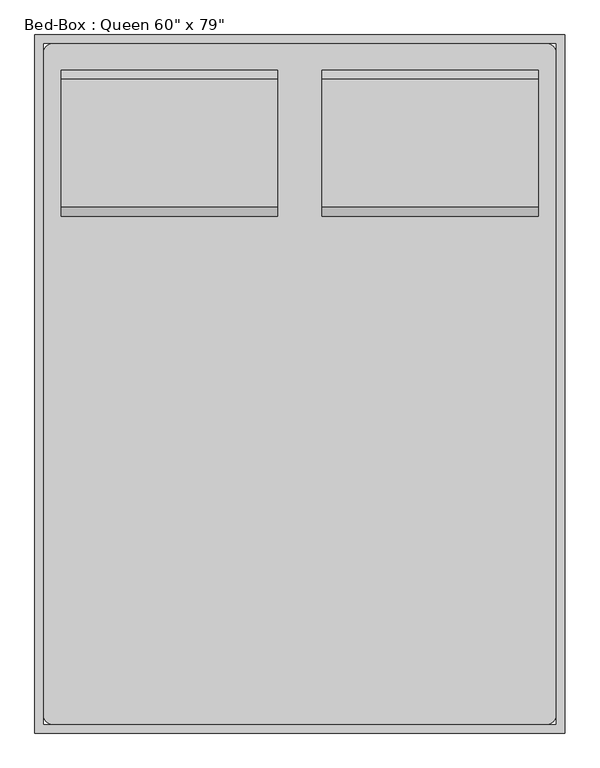
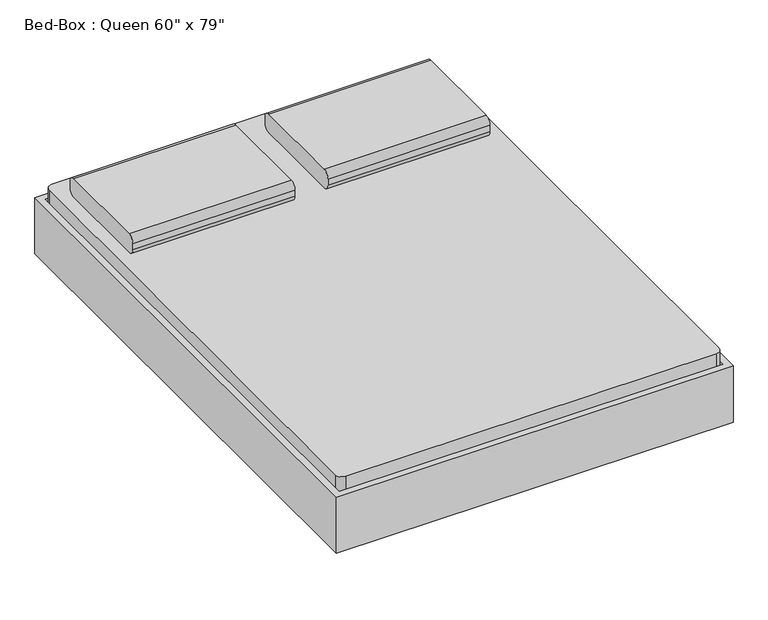
"""IFC4 building model written with IfcOpenShell, lengths in millimetres: furniture geometry."""

from ifc_helpers import new_model, si_unit, point, frame, frame_2d, origin, place, context, project, spatial, polyline, circle_curve, trimmed, segment, composite_curve, outline, extrude, source, transform, mapped, element, save
from ifc_brep_helpers import plane_surface, cylinder_surface, revolved_surface, advanced_brep


def furniture_1d2926bd(model_context):
    return source(origin(), model_context, "Body", "SolidModel", [
        extrude(outline(composite_curve([segment(polyline([(641.8704918, 406.4), (273.5704918, 406.4)]), True, "CONTINUOUS"), segment(trimmed(circle_curve(frame_2d((273.5704918, 431.8)), 25.4), [point((273.5704918, 406.4))], [point((248.1704918, 431.8))], False, "CARTESIAN"), True, "CONTINUOUS"), segment(polyline([(248.1704918, 431.8), (248.1704918, 457.2)]), True, "CONTINUOUS"), segment(trimmed(circle_curve(frame_2d((273.5704918, 457.2)), 25.4), [point((248.1704918, 457.2))], [point((273.5704918, 482.6))], False, "CARTESIAN"), True, "CONTINUOUS"), segment(polyline([(273.5704918, 482.6), (641.8704918, 482.6)]), True, "CONTINUOUS"), segment(trimmed(circle_curve(frame_2d((641.8704918, 457.2)), 25.4), [point((641.8704918, 482.6))], [point((667.2704918, 457.2))], False, "CARTESIAN"), True, "CONTINUOUS"), segment(polyline([(667.2704918, 457.2), (667.2704918, 431.8)]), True, "CONTINUOUS"), segment(trimmed(circle_curve(frame_2d((641.8704918, 431.8)), 25.4), [point((667.2704918, 431.8))], [point((641.8704918, 406.4))], False, "CARTESIAN"), True, "CONTINUOUS")], self_intersect=False)), frame((402.652459, 0.0, 0.0), z_axis=(1.0, 0.0, 0.0), x_axis=(0.0, 1.0, 0.0)), (0.0, 0.0, 1.0), 622.3),
        extrude(outline(composite_curve([segment(polyline([(641.8704918, 406.4), (273.5704918, 406.4)]), True, "CONTINUOUS"), segment(trimmed(circle_curve(frame_2d((273.5704918, 431.8)), 25.4), [point((273.5704918, 406.4))], [point((248.1704918, 431.8))], False, "CARTESIAN"), True, "CONTINUOUS"), segment(polyline([(248.1704918, 431.8), (248.1704918, 457.2)]), True, "CONTINUOUS"), segment(trimmed(circle_curve(frame_2d((273.5704918, 457.2)), 25.4), [point((248.1704918, 457.2))], [point((273.5704918, 482.6))], False, "CARTESIAN"), True, "CONTINUOUS"), segment(polyline([(273.5704918, 482.6), (641.8704918, 482.6)]), True, "CONTINUOUS"), segment(trimmed(circle_curve(frame_2d((641.8704918, 457.2)), 25.4), [point((641.8704918, 482.6))], [point((667.2704918, 457.2))], False, "CARTESIAN"), True, "CONTINUOUS"), segment(polyline([(667.2704918, 457.2), (667.2704918, 431.8)]), True, "CONTINUOUS"), segment(trimmed(circle_curve(frame_2d((641.8704918, 431.8)), 25.4), [point((667.2704918, 431.8))], [point((641.8704918, 406.4))], False, "CARTESIAN"), True, "CONTINUOUS")], self_intersect=False)), frame((-346.647541, 0.0, 0.0), z_axis=(1.0, 0.0, 0.0), x_axis=(0.0, 1.0, 0.0)), (0.0, 0.0, 1.0), 622.3),
        advanced_brep(
        [(-397.1231784, 514.8704918, 177.8), (-397.1231784, 438.6704918, 177.8), (-397.1231784, 438.6704918, 196.85), (-397.1231784, 514.8704918, 196.85), (-346.3231784, 514.8704918, 177.8), (-346.3231784, 438.6704918, 177.8), (-334.1869899, 438.6704918, 196.85), (-334.1869899, 514.8704918, 196.85), (-270.2523099, 514.8704918, 14.6654962), (-270.2523099, 438.6704918, 14.6654962), (-252.9871466, 438.6704918, 22.716374), (-252.9871466, 514.8704918, 22.716374), (-247.2320921, 438.6704918, 0.0), (-247.2320921, 514.8704918, 0.0), (-247.2320921, 438.6704918, 19.05), (-247.2320921, 514.8704918, 19.05), (-168.6195862, 514.8704918, 0.0), (-168.6195862, 438.6704918, 0.0), (-168.6195862, 438.6704918, 19.05), (-168.6195862, 514.8704918, 19.05), (-155.9195862, 438.6704918, 3.4029547), (-155.9195862, 514.8704918, 3.4029547), (-165.4445862, 438.6704918, 19.9007387), (-165.4445862, 514.8704918, 19.9007387), (-95.822541, 514.8704918, 38.1), (-95.822541, 438.6704918, 38.1), (-100.9269731, 438.6704918, 57.15), (-100.9269731, 514.8704918, 57.15), (774.4518216, 514.8704918, 38.1), (774.4518216, 438.6704918, 38.1), (779.5562537, 438.6704918, 57.15), (779.5562537, 514.8704918, 57.15), (834.5488669, 514.8704918, 3.4029547), (834.5488669, 438.6704918, 3.4029547), (844.0738669, 438.6704918, 19.9007387), (844.0738669, 514.8704918, 19.9007387), (847.2488669, 438.6704918, 0.0), (847.2488669, 514.8704918, 0.0), (847.2488669, 438.6704918, 19.05), (847.2488669, 514.8704918, 19.05), (925.8613728, 514.8704918, 0.0), (925.8613728, 438.6704918, 0.0), (925.8613728, 438.6704918, 19.05), (925.8613728, 514.8704918, 19.05), (948.8815906, 438.6704918, 14.6654962), (948.8815906, 514.8704918, 14.6654962), (931.6164272, 438.6704918, 22.716374), (931.6164272, 514.8704918, 22.716374), (1024.952459, 514.8704918, 177.8), (1024.952459, 438.6704918, 177.8), (1012.8162705, 438.6704918, 196.85), (1012.8162705, 514.8704918, 196.85), (1075.752459, 514.8704918, 177.8), (1075.752459, 514.8704918, 196.85), (1075.752459, 438.6704918, 196.85), (1075.752459, 438.6704918, 177.8)],
        [
            (0, 1),
            (1, 2),
            (2, 3),
            (3, 0),
            (0, 4),
            (4, 5),
            (5, 1),
            (5, 6),
            (6, 2),
            (6, 7),
            (7, 3),
            (7, 4),
            (4, 8),
            (8, 9),
            (9, 5),
            (9, 10),
            (10, 6),
            (10, 11),
            (11, 7),
            (11, 8),
            (12, 9, circle_curve(frame((-247.2320921, 438.6704918, 25.4), z_axis=(0.0, 1.0, 0.0), x_axis=(-0.9063077870366486, 0.0, -0.42261826174070233)), 25.4)),
            (8, 13, circle_curve(frame((-247.2320921, 514.8704918, 25.4), z_axis=(0.0, -1.0, 0.0), x_axis=(-0.9063077870366486, 0.0, -0.42261826174070233)), 25.4)),
            (13, 12),
            (14, 10, circle_curve(frame((-247.2320921, 438.6704918, 25.4), z_axis=(0.0, 1.0, 0.0), x_axis=(-0.9063077870366486, 0.0, -0.42261826174070233)), 6.35)),
            (12, 14),
            (15, 11, circle_curve(frame((-247.2320921, 514.8704918, 25.4), z_axis=(0.0, 1.0, 0.0), x_axis=(-0.9063077870366486, 0.0, -0.42261826174070233)), 6.35)),
            (14, 15),
            (15, 13),
            (13, 16),
            (16, 17),
            (17, 12),
            (17, 18),
            (18, 14),
            (18, 19),
            (19, 15),
            (19, 16),
            (20, 17, circle_curve(frame((-168.6195862, 438.6704918, 25.4), z_axis=(0.0, 1.0, 0.0), x_axis=(0.0, 0.0, -1.0)), 25.4)),
            (16, 21, circle_curve(frame((-168.6195862, 514.8704918, 25.4), z_axis=(0.0, -1.0, 0.0), x_axis=(0.0, 0.0, -1.0)), 25.4)),
            (21, 20),
            (22, 18, circle_curve(frame((-168.6195862, 438.6704918, 25.4), z_axis=(0.0, 1.0, 0.0), x_axis=(0.0, 0.0, -1.0)), 6.35)),
            (20, 22),
            (23, 19, circle_curve(frame((-168.6195862, 514.8704918, 25.4), z_axis=(0.0, 1.0, 0.0), x_axis=(0.0, 0.0, -1.0)), 6.35)),
            (22, 23),
            (23, 21),
            (21, 24),
            (24, 25),
            (25, 20),
            (25, 26),
            (26, 22),
            (26, 27),
            (27, 23),
            (27, 24),
            (24, 28),
            (28, 29),
            (29, 25),
            (29, 30),
            (30, 26),
            (30, 31),
            (31, 27),
            (31, 28),
            (28, 32),
            (32, 33),
            (33, 29),
            (33, 34),
            (34, 30),
            (34, 35),
            (35, 31),
            (35, 32),
            (36, 33, circle_curve(frame((847.2488669, 438.6704918, 25.4), z_axis=(0.0, 1.0, 0.0), x_axis=(-0.5000000000000463, 0.0, -0.8660254037844118)), 25.4)),
            (32, 37, circle_curve(frame((847.2488669, 514.8704918, 25.4), z_axis=(0.0, -1.0, 0.0), x_axis=(-0.5000000000000463, 0.0, -0.8660254037844118)), 25.4)),
            (37, 36),
            (38, 34, circle_curve(frame((847.2488669, 438.6704918, 25.4), z_axis=(0.0, 1.0, 0.0), x_axis=(-0.5000000000000463, 0.0, -0.8660254037844118)), 6.35)),
            (36, 38),
            (39, 35, circle_curve(frame((847.2488669, 514.8704918, 25.4), z_axis=(0.0, 1.0, 0.0), x_axis=(-0.5000000000000463, 0.0, -0.8660254037844118)), 6.35)),
            (38, 39),
            (39, 37),
            (37, 40),
            (40, 41),
            (41, 36),
            (41, 42),
            (42, 38),
            (42, 43),
            (43, 39),
            (43, 40),
            (44, 41, circle_curve(frame((925.8613728, 438.6704918, 25.4), z_axis=(0.0, 1.0, 0.0), x_axis=(0.0, 0.0, -1.0)), 25.4)),
            (40, 45, circle_curve(frame((925.8613728, 514.8704918, 25.4), z_axis=(0.0, -1.0, 0.0), x_axis=(0.0, 0.0, -1.0)), 25.4)),
            (45, 44),
            (46, 42, circle_curve(frame((925.8613728, 438.6704918, 25.4), z_axis=(0.0, 1.0, 0.0), x_axis=(0.0, 0.0, -1.0)), 6.35)),
            (44, 46),
            (47, 43, circle_curve(frame((925.8613728, 514.8704918, 25.4), z_axis=(0.0, 1.0, 0.0), x_axis=(0.0, 0.0, -1.0)), 6.35)),
            (46, 47),
            (47, 45),
            (45, 48),
            (48, 49),
            (49, 44),
            (49, 50),
            (50, 46),
            (50, 51),
            (51, 47),
            (51, 48),
            (52, 53),
            (53, 54),
            (54, 55),
            (55, 52),
            (48, 52),
            (55, 49),
            (54, 50),
            (53, 51),
        ],
        [
            plane_surface(frame((-397.1231784, 768.8704918, -152.9490627), z_axis=(-1.0, 0.0, 0.0), x_axis=(0.0, 1.0, 0.0))),
            plane_surface(frame((-397.1231784, 514.8704918, 177.8), z_axis=(0.0, 0.0, -1.0), x_axis=(1.0, 0.0, 0.0))),
            plane_surface(frame((-397.1231784, 438.6704918, 177.8), z_axis=(0.0, -1.0, 0.0), x_axis=(1.0, 0.0, 0.0))),
            plane_surface(frame((-397.1231784, 438.6704918, 196.85), z_axis=(0.0, 0.0, 1.0), x_axis=(1.0, 0.0, 0.0))),
            plane_surface(frame((-397.1231784, 514.8704918, 196.85), z_axis=(0.0, 1.0, 0.0), x_axis=(1.0, 0.0, 0.0))),
            plane_surface(frame((-346.3231784, 514.8704918, 177.8), z_axis=(-0.9063077870366485, 0.0, -0.4226182617407027), x_axis=(0.4226182617407027, 0.0, -0.9063077870366485))),
            plane_surface(frame((-346.3231784, 438.6704918, 177.8), z_axis=(0.0, -1.0, 0.0), x_axis=(0.4226182617407025, 0.0, -0.9063077870366486))),
            plane_surface(frame((-334.1869899, 438.6704918, 196.85), z_axis=(0.9063077870366484, 0.0, 0.4226182617407028), x_axis=(0.4226182617407028, 0.0, -0.9063077870366484))),
            plane_surface(frame((-334.1869899, 514.8704918, 196.85), z_axis=(0.0, 1.0, 0.0), x_axis=(0.42261826174070277, 0.0, -0.9063077870366485))),
            cylinder_surface(frame((-247.2320921, 768.8704918, 25.4), z_axis=(0.0, -1.0, 0.0), x_axis=(-0.9063077870366486, 0.0, -0.42261826174070233)), 25.4),
            plane_surface(frame((-247.2320921, 438.6704918, 25.4), z_axis=(0.0, -1.0, 0.0), x_axis=(-0.9063077870366486, 0.0, -0.42261826174070233))),
            revolved_surface(polyline([(-252.9871465476827, 438.6704918, 22.71637403794654), (-252.9871465476827, 514.8704918, 22.71637403794654)]), (-247.2320921, 768.8704918, 25.4), (0.0, -1.0, 0.0)),
            plane_surface(frame((-247.2320921, 514.8704918, 25.4), z_axis=(0.0, 1.0, 0.0), x_axis=(-0.9063077870366486, 0.0, -0.42261826174070233))),
            plane_surface(frame((-247.2320921, 514.8704918, 0.0), z_axis=(0.0, 0.0, -1.0), x_axis=(1.0, 0.0, 0.0))),
            plane_surface(frame((-247.2320921, 438.6704918, 0.0), z_axis=(0.0, -1.0, 0.0), x_axis=(1.0, 0.0, 0.0))),
            plane_surface(frame((-247.2320921, 438.6704918, 19.05), z_axis=(0.0, 0.0, 1.0), x_axis=(1.0, 0.0, 0.0))),
            plane_surface(frame((-247.2320921, 514.8704918, 19.05), z_axis=(0.0, 1.0, 0.0), x_axis=(1.0, 0.0, 0.0))),
            cylinder_surface(frame((-168.6195862, 768.8704918, 25.4), z_axis=(0.0, -1.0, 0.0), x_axis=(0.0, 0.0, -1.0)), 25.4),
            plane_surface(frame((-168.6195862, 438.6704918, 25.4), z_axis=(0.0, -1.0, 0.0), x_axis=(0.0, 0.0, -1.0))),
            revolved_surface(polyline([(-168.6195862, 438.6704918, 19.049999999999997), (-168.6195862, 514.8704918, 19.049999999999997)]), (-168.6195862, 768.8704918, 25.4), (0.0, -1.0, 0.0)),
            plane_surface(frame((-168.6195862, 514.8704918, 25.4), z_axis=(0.0, 1.0, 0.0), x_axis=(0.0, 0.0, -1.0))),
            plane_surface(frame((-155.9195862, 514.8704918, 3.4029547), z_axis=(0.49999999999988004, 0.0, -0.866025403784508), x_axis=(0.866025403784508, 0.0, 0.49999999999988004))),
            plane_surface(frame((-155.9195862, 438.6704918, 3.4029547), z_axis=(0.0, -1.0, 0.0), x_axis=(0.8660254037845078, 0.0, 0.49999999999988026))),
            plane_surface(frame((-165.4445862, 438.6704918, 19.9007387), z_axis=(-0.4999999999998799, 0.0, 0.866025403784508), x_axis=(0.866025403784508, 0.0, 0.4999999999998799))),
            plane_surface(frame((-165.4445862, 514.8704918, 19.9007387), z_axis=(0.0, 1.0, 0.0), x_axis=(0.8660254037845075, 0.0, 0.49999999999988076))),
            plane_surface(frame((-95.822541, 514.8704918, 38.1), z_axis=(0.0, 0.0, -1.0), x_axis=(1.0, 0.0, 0.0))),
            plane_surface(frame((-95.822541, 438.6704918, 38.1), z_axis=(0.0, -1.0, 0.0), x_axis=(1.0, 0.0, 0.0))),
            plane_surface(frame((-100.9269731, 438.6704918, 57.15), z_axis=(0.0, 0.0, 1.0), x_axis=(1.0, 0.0, 0.0))),
            plane_surface(frame((-100.9269731, 514.8704918, 57.15), z_axis=(0.0, 1.0, 0.0), x_axis=(1.0, 0.0, 0.0))),
            plane_surface(frame((774.4518216, 514.8704918, 38.1), z_axis=(-0.5000000000000455, 0.0, -0.8660254037844125), x_axis=(0.8660254037844125, 0.0, -0.5000000000000455))),
            plane_surface(frame((774.4518216, 438.6704918, 38.1), z_axis=(0.0, -1.0, 0.0), x_axis=(0.866025403784412, 0.0, -0.5000000000000463))),
            plane_surface(frame((779.5562537, 438.6704918, 57.15), z_axis=(0.5000000000000466, 0.0, 0.8660254037844117), x_axis=(0.8660254037844117, 0.0, -0.5000000000000466))),
            plane_surface(frame((779.5562537, 514.8704918, 57.15), z_axis=(0.0, 1.0, 0.0), x_axis=(0.8660254037844115, 0.0, -0.5000000000000471))),
            cylinder_surface(frame((847.2488669, 768.8704918, 25.4), z_axis=(0.0, -1.0, 0.0), x_axis=(-0.5000000000000463, 0.0, -0.8660254037844118)), 25.4),
            plane_surface(frame((847.2488669, 438.6704918, 25.4), z_axis=(0.0, -1.0000000000000002, 0.0), x_axis=(-0.5000000000000464, 0.0, -0.866025403784412))),
            revolved_surface(polyline([(844.0738668999998, 438.6704918, 19.90073868596898), (844.0738668999998, 514.8704918, 19.90073868596898)]), (847.2488669, 768.8704918, 25.4), (0.0, -1.0, 0.0)),
            plane_surface(frame((847.2488669, 514.8704918, 25.4), z_axis=(0.0, 1.0000000000000002, 0.0), x_axis=(-0.5000000000000464, 0.0, -0.866025403784412))),
            plane_surface(frame((847.2488669, 514.8704918, 0.0), z_axis=(0.0, 0.0, -1.0), x_axis=(1.0, 0.0, 0.0))),
            plane_surface(frame((847.2488669, 438.6704918, 0.0), z_axis=(0.0, -1.0, 0.0), x_axis=(1.0, 0.0, 0.0))),
            plane_surface(frame((847.2488669, 438.6704918, 19.05), z_axis=(0.0, 0.0, 1.0), x_axis=(1.0, 0.0, 0.0))),
            plane_surface(frame((847.2488669, 514.8704918, 19.05), z_axis=(0.0, 1.0, 0.0), x_axis=(1.0, 0.0, 0.0))),
            cylinder_surface(frame((925.8613728, 768.8704918, 25.4), z_axis=(0.0, -1.0, 0.0), x_axis=(0.0, 0.0, -1.0)), 25.4),
            plane_surface(frame((925.8613728, 438.6704918, 25.4), z_axis=(0.0, -1.0, 0.0), x_axis=(0.0, 0.0, -1.0))),
            revolved_surface(polyline([(925.8613728, 438.6704918, 19.049999999999997), (925.8613728, 514.8704918, 19.049999999999997)]), (925.8613728, 768.8704918, 25.4), (0.0, -1.0, 0.0)),
            plane_surface(frame((925.8613728, 514.8704918, 25.4), z_axis=(0.0, 1.0, 0.0), x_axis=(0.0, 0.0, -1.0))),
            plane_surface(frame((948.8815906, 514.8704918, 14.6654962), z_axis=(0.90630778703668, 0.0, -0.42261826174063505), x_axis=(0.42261826174063505, 0.0, 0.90630778703668))),
            plane_surface(frame((948.8815906, 438.6704918, 14.6654962), z_axis=(0.0, -1.0, 0.0), x_axis=(0.42261826174063566, 0.0, 0.9063077870366797))),
            plane_surface(frame((931.6164272, 438.6704918, 22.716374), z_axis=(-0.9063077870366801, 0.0, 0.42261826174063477), x_axis=(0.42261826174063477, 0.0, 0.9063077870366801))),
            plane_surface(frame((931.6164272, 514.8704918, 22.716374), z_axis=(0.0, 1.0, 0.0), x_axis=(0.4226182617406345, 0.0, 0.9063077870366802))),
            plane_surface(frame((1075.752459, 768.8704918, -152.9490627), z_axis=(1.0, 0.0, 0.0), x_axis=(0.0, 1.0, 0.0))),
            plane_surface(frame((1024.952459, 514.8704918, 177.8), z_axis=(0.0, 0.0, -1.0), x_axis=(1.0, 0.0, 0.0))),
            plane_surface(frame((1024.952459, 438.6704918, 177.8), z_axis=(0.0, -1.0, 0.0), x_axis=(1.0, 0.0, 0.0))),
            plane_surface(frame((1012.8162705, 438.6704918, 196.85), z_axis=(0.0, 0.0, 1.0), x_axis=(1.0, 0.0, 0.0))),
            plane_surface(frame((1012.8162705, 514.8704918, 196.85), z_axis=(0.0, 1.0, 0.0), x_axis=(1.0, 0.0, 0.0))),
        ],
        [
            (0, [[1, 2, 3, 4]]),
            (1, [[-1, 5, 6, 7]]),
            (2, [[-2, -7, 8, 9]]),
            (3, [[-3, -9, 10, 11]]),
            (4, [[-4, -11, 12, -5]]),
            (5, [[-6, 13, 14, 15]]),
            (6, [[-8, -15, 16, 17]]),
            (7, [[-10, -17, 18, 19]]),
            (8, [[-12, -19, 20, -13]]),
            (9, [[21, -14, 22, 23]]),
            (10, [[24, -16, -21, 25]]),
            (11, [[26, -18, -24, 27]]),
            (12, [[-22, -20, -26, 28]]),
            (13, [[-23, 29, 30, 31]]),
            (14, [[-25, -31, 32, 33]]),
            (15, [[-27, -33, 34, 35]]),
            (16, [[-28, -35, 36, -29]]),
            (17, [[37, -30, 38, 39]]),
            (18, [[40, -32, -37, 41]]),
            (19, [[42, -34, -40, 43]]),
            (20, [[-38, -36, -42, 44]]),
            (21, [[-39, 45, 46, 47]]),
            (22, [[-41, -47, 48, 49]]),
            (23, [[-43, -49, 50, 51]]),
            (24, [[-44, -51, 52, -45]]),
            (25, [[-46, 53, 54, 55]]),
            (26, [[-48, -55, 56, 57]]),
            (27, [[-50, -57, 58, 59]]),
            (28, [[-52, -59, 60, -53]]),
            (29, [[-54, 61, 62, 63]]),
            (30, [[-56, -63, 64, 65]]),
            (31, [[-58, -65, 66, 67]]),
            (32, [[-60, -67, 68, -61]]),
            (33, [[69, -62, 70, 71]]),
            (34, [[72, -64, -69, 73]]),
            (35, [[74, -66, -72, 75]]),
            (36, [[-70, -68, -74, 76]]),
            (37, [[-71, 77, 78, 79]]),
            (38, [[-73, -79, 80, 81]]),
            (39, [[-75, -81, 82, 83]]),
            (40, [[-76, -83, 84, -77]]),
            (41, [[85, -78, 86, 87]]),
            (42, [[88, -80, -85, 89]]),
            (43, [[90, -82, -88, 91]]),
            (44, [[-86, -84, -90, 92]]),
            (45, [[-87, 93, 94, 95]]),
            (46, [[-89, -95, 96, 97]]),
            (47, [[-91, -97, 98, 99]]),
            (48, [[-92, -99, 100, -93]]),
            (49, [[101, 102, 103, 104]]),
            (50, [[-94, 105, -104, 106]]),
            (51, [[-96, -106, -103, 107]]),
            (52, [[-98, -107, -102, 108]]),
            (53, [[-100, -108, -101, -105]]),
        ],
    ),
        extrude(outline(composite_curve([segment(polyline([(-372.047541, 743.4704918), (1050.352459, 743.4704918)]), True, "CONTINUOUS"), segment(trimmed(circle_curve(frame_2d((1050.352459, 718.0704918)), 25.4), [point((1050.352459, 743.4704918))], [point((1075.752459, 718.0704918))], False, "CARTESIAN"), True, "CONTINUOUS"), segment(polyline([(1075.752459, 718.0704918), (1075.752459, -1186.9295082)]), True, "CONTINUOUS"), segment(trimmed(circle_curve(frame_2d((1050.352459, -1186.9295082)), 25.4), [point((1075.752459, -1186.9295082))], [point((1050.352459, -1212.3295082))], False, "CARTESIAN"), True, "CONTINUOUS"), segment(polyline([(1050.352459, -1212.3295082), (-372.047541, -1212.3295082)]), True, "CONTINUOUS"), segment(trimmed(circle_curve(frame_2d((-372.047541, -1186.9295082)), 25.4), [point((-372.047541, -1212.3295082))], [point((-397.447541, -1186.9295082))], False, "CARTESIAN"), True, "CONTINUOUS"), segment(polyline([(-397.447541, -1186.9295082), (-397.447541, 718.0704918)]), True, "CONTINUOUS"), segment(trimmed(circle_curve(frame_2d((-372.047541, 718.0704918)), 25.4), [point((-397.447541, 718.0704918))], [point((-372.047541, 743.4704918))], False, "CARTESIAN"), True, "CONTINUOUS")], self_intersect=False)), frame((0.0, 0.0, 203.2), z_axis=(0.0, 0.0, 1.0), x_axis=(1.0, 0.0, 0.0)), (0.0, 0.0, 1.0), 203.2),
        advanced_brep(
        [(-397.447541, -932.9295082, 196.85), (-397.447541, -932.9295082, 177.8), (-397.447541, -1009.1295082, 177.8), (-397.447541, -1009.1295082, 196.85), (-334.5113525, -932.9295082, 196.85), (-346.647541, -932.9295082, 177.8), (-346.647541, -1009.1295082, 177.8), (-334.5113525, -1009.1295082, 196.85), (-253.3115092, -932.9295082, 22.716374), (-270.5766725, -932.9295082, 14.6654962), (-270.5766725, -1009.1295082, 14.6654962), (-253.3115092, -1009.1295082, 22.716374), (-247.5564547, -932.9295082, 0.0), (-247.5564547, -932.9295082, 19.05), (-247.5564547, -1009.1295082, 0.0), (-247.5564547, -1009.1295082, 19.05), (-168.9439489, -932.9295082, 19.05), (-168.9439489, -932.9295082, 0.0), (-168.9439489, -1009.1295082, 0.0), (-168.9439489, -1009.1295082, 19.05), (-156.2439489, -932.9295082, 3.4029547), (-165.7689489, -932.9295082, 19.9007387), (-156.2439489, -1009.1295082, 3.4029547), (-165.7689489, -1009.1295082, 19.9007387), (-101.2513357, -932.9295082, 57.15), (-96.1469036, -932.9295082, 38.1), (-96.1469036, -1009.1295082, 38.1), (-101.2513357, -1009.1295082, 57.15), (779.5562537, -932.9295082, 57.15), (774.4518216, -932.9295082, 38.1), (774.4518216, -1009.1295082, 38.1), (779.5562537, -1009.1295082, 57.15), (844.0738669, -932.9295082, 19.9007387), (834.5488669, -932.9295082, 3.4029547), (834.5488669, -1009.1295082, 3.4029547), (844.0738669, -1009.1295082, 19.9007387), (847.2488669, -932.9295082, 0.0), (847.2488669, -932.9295082, 19.05), (847.2488669, -1009.1295082, 0.0), (847.2488669, -1009.1295082, 19.05), (925.8613728, -932.9295082, 19.05), (925.8613728, -932.9295082, 0.0), (925.8613728, -1009.1295082, 0.0), (925.8613728, -1009.1295082, 19.05), (948.8815906, -932.9295082, 14.6654962), (931.6164272, -932.9295082, 22.716374), (948.8815906, -1009.1295082, 14.6654962), (931.6164272, -1009.1295082, 22.716374), (1012.8162705, -932.9295082, 196.85), (1024.952459, -932.9295082, 177.8), (1024.952459, -1009.1295082, 177.8), (1012.8162705, -1009.1295082, 196.85), (1075.752459, -932.9295082, 196.85), (1075.752459, -1009.1295082, 196.85), (1075.752459, -1009.1295082, 177.8), (1075.752459, -932.9295082, 177.8)],
        [
            (0, 1),
            (1, 2),
            (2, 3),
            (3, 0),
            (0, 4),
            (4, 5),
            (5, 1),
            (5, 6),
            (6, 2),
            (6, 7),
            (7, 3),
            (7, 4),
            (4, 8),
            (8, 9),
            (9, 5),
            (9, 10),
            (10, 6),
            (10, 11),
            (11, 7),
            (11, 8),
            (12, 9, circle_curve(frame((-247.5564547, -932.9295082, 25.4), z_axis=(0.0, 1.0, 0.0), x_axis=(-0.906307787036663, 0.0, -0.4226182617406713)), 25.4)),
            (8, 13, circle_curve(frame((-247.5564547, -932.9295082, 25.4), z_axis=(0.0, -1.0, 0.0), x_axis=(-0.906307787036663, 0.0, -0.4226182617406713)), 6.35)),
            (13, 12),
            (14, 10, circle_curve(frame((-247.5564547, -1009.1295082, 25.4), z_axis=(0.0, 1.0, 0.0), x_axis=(-0.906307787036663, 0.0, -0.4226182617406713)), 25.4)),
            (12, 14),
            (15, 11, circle_curve(frame((-247.5564547, -1009.1295082, 25.4), z_axis=(0.0, 1.0, 0.0), x_axis=(-0.906307787036663, 0.0, -0.4226182617406713)), 6.35)),
            (14, 15),
            (15, 13),
            (13, 16),
            (16, 17),
            (17, 12),
            (17, 18),
            (18, 14),
            (18, 19),
            (19, 15),
            (19, 16),
            (20, 17, circle_curve(frame((-168.9439489, -932.9295082, 25.4), z_axis=(0.0, 1.0, 0.0), x_axis=(0.0, 0.0, -1.0)), 25.4)),
            (16, 21, circle_curve(frame((-168.9439489, -932.9295082, 25.4), z_axis=(0.0, -1.0, 0.0), x_axis=(0.0, 0.0, -1.0)), 6.35)),
            (21, 20),
            (22, 18, circle_curve(frame((-168.9439489, -1009.1295082, 25.4), z_axis=(0.0, 1.0, 0.0), x_axis=(0.0, 0.0, -1.0)), 25.4)),
            (20, 22),
            (23, 19, circle_curve(frame((-168.9439489, -1009.1295082, 25.4), z_axis=(0.0, 1.0, 0.0), x_axis=(0.0, 0.0, -1.0)), 6.35)),
            (22, 23),
            (23, 21),
            (21, 24),
            (24, 25),
            (25, 20),
            (25, 26),
            (26, 22),
            (26, 27),
            (27, 23),
            (27, 24),
            (24, 28),
            (28, 29),
            (29, 25),
            (29, 30),
            (30, 26),
            (30, 31),
            (31, 27),
            (31, 28),
            (28, 32),
            (32, 33),
            (33, 29),
            (33, 34),
            (34, 30),
            (34, 35),
            (35, 31),
            (35, 32),
            (36, 33, circle_curve(frame((847.2488669, -932.9295082, 25.4), z_axis=(0.0, 1.0, 0.0), x_axis=(-0.5000000000000479, 0.0, -0.866025403784411)), 25.4)),
            (32, 37, circle_curve(frame((847.2488669, -932.9295082, 25.4), z_axis=(0.0, -1.0, 0.0), x_axis=(-0.5000000000000479, 0.0, -0.866025403784411)), 6.35)),
            (37, 36),
            (38, 34, circle_curve(frame((847.2488669, -1009.1295082, 25.4), z_axis=(0.0, 1.0, 0.0), x_axis=(-0.5000000000000479, 0.0, -0.866025403784411)), 25.4)),
            (36, 38),
            (39, 35, circle_curve(frame((847.2488669, -1009.1295082, 25.4), z_axis=(0.0, 1.0, 0.0), x_axis=(-0.5000000000000479, 0.0, -0.866025403784411)), 6.35)),
            (38, 39),
            (39, 37),
            (37, 40),
            (40, 41),
            (41, 36),
            (41, 42),
            (42, 38),
            (42, 43),
            (43, 39),
            (43, 40),
            (44, 41, circle_curve(frame((925.8613728, -932.9295082, 25.4), z_axis=(0.0, 1.0, 0.0), x_axis=(0.0, 0.0, -1.0)), 25.4)),
            (40, 45, circle_curve(frame((925.8613728, -932.9295082, 25.4), z_axis=(0.0, -1.0, 0.0), x_axis=(0.0, 0.0, -1.0)), 6.35)),
            (45, 44),
            (46, 42, circle_curve(frame((925.8613728, -1009.1295082, 25.4), z_axis=(0.0, 1.0, 0.0), x_axis=(0.0, 0.0, -1.0)), 25.4)),
            (44, 46),
            (47, 43, circle_curve(frame((925.8613728, -1009.1295082, 25.4), z_axis=(0.0, 1.0, 0.0), x_axis=(0.0, 0.0, -1.0)), 6.35)),
            (46, 47),
            (47, 45),
            (45, 48),
            (48, 49),
            (49, 44),
            (49, 50),
            (50, 46),
            (50, 51),
            (51, 47),
            (51, 48),
            (52, 53),
            (53, 54),
            (54, 55),
            (55, 52),
            (48, 52),
            (55, 49),
            (54, 50),
            (53, 51),
        ],
        [
            plane_surface(frame((-397.447541, -1237.7295082, -127.5947323), z_axis=(-1.0, 0.0, 0.0), x_axis=(0.0, 1.0, 0.0))),
            plane_surface(frame((-397.447541, -932.9295082, 196.85), z_axis=(0.0, 1.0, 0.0), x_axis=(1.0, 0.0, 0.0))),
            plane_surface(frame((-397.447541, -932.9295082, 177.8), z_axis=(0.0, 0.0, -1.0), x_axis=(1.0, 0.0, 0.0))),
            plane_surface(frame((-397.447541, -1009.1295082, 177.8), z_axis=(0.0, -1.0, 0.0), x_axis=(1.0, 0.0, 0.0))),
            plane_surface(frame((-397.447541, -1009.1295082, 196.85), z_axis=(0.0, 0.0, 1.0), x_axis=(1.0, 0.0, 0.0))),
            plane_surface(frame((-334.5113525, -932.9295082, 196.85), z_axis=(0.0, 1.0, 0.0), x_axis=(0.4226182617406707, 0.0, -0.9063077870366634))),
            plane_surface(frame((-346.647541, -932.9295082, 177.8), z_axis=(-0.9063077870366635, 0.0, -0.4226182617406707), x_axis=(0.4226182617406707, 0.0, -0.9063077870366635))),
            plane_surface(frame((-346.647541, -1009.1295082, 177.8), z_axis=(0.0, -1.0, 0.0), x_axis=(0.422618261740671, 0.0, -0.9063077870366633))),
            plane_surface(frame((-334.5113525, -1009.1295082, 196.85), z_axis=(0.9063077870366633, 0.0, 0.42261826174067113), x_axis=(0.42261826174067113, 0.0, -0.9063077870366633))),
            plane_surface(frame((-247.5564547, -932.9295082, 25.4), z_axis=(0.0, 1.0, 0.0), x_axis=(-0.906307787036663, 0.0, -0.4226182617406713))),
            cylinder_surface(frame((-247.5564547, -1237.7295082, 25.4), z_axis=(0.0, -1.0, 0.0), x_axis=(-0.906307787036663, 0.0, -0.4226182617406713)), 25.4),
            plane_surface(frame((-247.5564547, -1009.1295082, 25.4), z_axis=(0.0, -1.0, 0.0), x_axis=(-0.906307787036663, 0.0, -0.4226182617406713))),
            revolved_surface(polyline([(-253.3115091476828, -1009.1295082, 22.716374037946736), (-253.3115091476828, -932.9295082, 22.716374037946736)]), (-247.5564547, -1237.7295082, 25.4), (0.0, -1.0, 0.0)),
            plane_surface(frame((-247.5564547, -932.9295082, 19.05), z_axis=(0.0, 1.0, 0.0), x_axis=(1.0, 0.0, 0.0))),
            plane_surface(frame((-247.5564547, -932.9295082, 0.0), z_axis=(0.0, 0.0, -1.0), x_axis=(1.0, 0.0, 0.0))),
            plane_surface(frame((-247.5564547, -1009.1295082, 0.0), z_axis=(0.0, -1.0, 0.0), x_axis=(1.0, 0.0, 0.0))),
            plane_surface(frame((-247.5564547, -1009.1295082, 19.05), z_axis=(0.0, 0.0, 1.0), x_axis=(1.0, 0.0, 0.0))),
            plane_surface(frame((-168.9439489, -932.9295082, 25.4), z_axis=(0.0, 1.0, 0.0), x_axis=(0.0, 0.0, -1.0))),
            cylinder_surface(frame((-168.9439489, -1237.7295082, 25.4), z_axis=(0.0, -1.0, 0.0), x_axis=(0.0, 0.0, -1.0)), 25.4),
            plane_surface(frame((-168.9439489, -1009.1295082, 25.4), z_axis=(0.0, -1.0, 0.0), x_axis=(0.0, 0.0, -1.0))),
            revolved_surface(polyline([(-168.9439489, -1009.1295082, 19.049999999999997), (-168.9439489, -932.9295082, 19.049999999999997)]), (-168.9439489, -1237.7295082, 25.4), (0.0, -1.0, 0.0)),
            plane_surface(frame((-165.7689489, -932.9295082, 19.9007387), z_axis=(0.0, 1.0, 0.0), x_axis=(0.8660254037844788, 0.0, 0.4999999999999306))),
            plane_surface(frame((-156.2439489, -932.9295082, 3.4029547), z_axis=(0.49999999999993017, 0.0, -0.866025403784479), x_axis=(0.866025403784479, 0.0, 0.49999999999993017))),
            plane_surface(frame((-156.2439489, -1009.1295082, 3.4029547), z_axis=(0.0, -1.0, 0.0), x_axis=(0.8660254037844785, 0.0, 0.49999999999993106))),
            plane_surface(frame((-165.7689489, -1009.1295082, 19.9007387), z_axis=(-0.4999999999999309, 0.0, 0.8660254037844786), x_axis=(0.8660254037844786, 0.0, 0.4999999999999309))),
            plane_surface(frame((-101.2513357, -932.9295082, 57.15), z_axis=(0.0, 1.0, 0.0), x_axis=(1.0, 0.0, 0.0))),
            plane_surface(frame((-96.1469036, -932.9295082, 38.1), z_axis=(0.0, 0.0, -1.0), x_axis=(1.0, 0.0, 0.0))),
            plane_surface(frame((-96.1469036, -1009.1295082, 38.1), z_axis=(0.0, -1.0, 0.0), x_axis=(1.0, 0.0, 0.0))),
            plane_surface(frame((-101.2513357, -1009.1295082, 57.15), z_axis=(0.0, 0.0, 1.0), x_axis=(1.0, 0.0, 0.0))),
            plane_surface(frame((779.5562537, -932.9295082, 57.15), z_axis=(0.0, 1.0000000000000002, 0.0), x_axis=(0.8660254037844106, 0.0, -0.5000000000000487))),
            plane_surface(frame((774.4518216, -932.9295082, 38.1), z_axis=(-0.5000000000000477, 0.0, -0.8660254037844112), x_axis=(0.8660254037844112, 0.0, -0.5000000000000477))),
            plane_surface(frame((774.4518216, -1009.1295082, 38.1), z_axis=(0.0, -1.0000000000000002, 0.0), x_axis=(0.8660254037844105, 0.0, -0.500000000000049))),
            plane_surface(frame((779.5562537, -1009.1295082, 57.15), z_axis=(0.5000000000000498, 0.0, 0.8660254037844098), x_axis=(0.8660254037844098, 0.0, -0.5000000000000498))),
            plane_surface(frame((847.2488669, -932.9295082, 25.4), z_axis=(0.0, 1.0000000000000002, 0.0), x_axis=(-0.500000000000048, 0.0, -0.8660254037844111))),
            cylinder_surface(frame((847.2488669, -1237.7295082, 25.4), z_axis=(0.0, -1.0, 0.0), x_axis=(-0.5000000000000479, 0.0, -0.866025403784411)), 25.4),
            plane_surface(frame((847.2488669, -1009.1295082, 25.4), z_axis=(0.0, -1.0000000000000002, 0.0), x_axis=(-0.500000000000048, 0.0, -0.8660254037844111))),
            revolved_surface(polyline([(844.0738668999998, -1009.1295082, 19.90073868596899), (844.0738668999998, -932.9295082, 19.90073868596899)]), (847.2488669, -1237.7295082, 25.4), (0.0, -1.0, 0.0)),
            plane_surface(frame((847.2488669, -932.9295082, 19.05), z_axis=(0.0, 1.0, 0.0), x_axis=(1.0, 0.0, 0.0))),
            plane_surface(frame((847.2488669, -932.9295082, 0.0), z_axis=(0.0, 0.0, -1.0), x_axis=(1.0, 0.0, 0.0))),
            plane_surface(frame((847.2488669, -1009.1295082, 0.0), z_axis=(0.0, -1.0, 0.0), x_axis=(1.0, 0.0, 0.0))),
            plane_surface(frame((847.2488669, -1009.1295082, 19.05), z_axis=(0.0, 0.0, 1.0), x_axis=(1.0, 0.0, 0.0))),
            plane_surface(frame((925.8613728, -932.9295082, 25.4), z_axis=(0.0, 1.0, 0.0), x_axis=(0.0, 0.0, -1.0))),
            cylinder_surface(frame((925.8613728, -1237.7295082, 25.4), z_axis=(0.0, -1.0, 0.0), x_axis=(0.0, 0.0, -1.0)), 25.4),
            plane_surface(frame((925.8613728, -1009.1295082, 25.4), z_axis=(0.0, -1.0, 0.0), x_axis=(0.0, 0.0, -1.0))),
            revolved_surface(polyline([(925.8613728, -1009.1295082, 19.049999999999997), (925.8613728, -932.9295082, 19.049999999999997)]), (925.8613728, -1237.7295082, 25.4), (0.0, -1.0, 0.0)),
            plane_surface(frame((931.6164272, -932.9295082, 22.716374), z_axis=(0.0, 1.0, 0.0), x_axis=(0.4226182617405411, 0.0, 0.9063077870367238))),
            plane_surface(frame((948.8815906, -932.9295082, 14.6654962), z_axis=(0.9063077870367237, 0.0, -0.4226182617405414), x_axis=(0.4226182617405414, 0.0, 0.9063077870367237))),
            plane_surface(frame((948.8815906, -1009.1295082, 14.6654962), z_axis=(0.0, -1.0, 0.0), x_axis=(0.42261826174054123, 0.0, 0.9063077870367238))),
            plane_surface(frame((931.6164272, -1009.1295082, 22.716374), z_axis=(-0.9063077870367237, 0.0, 0.4226182617405414), x_axis=(0.4226182617405414, 0.0, 0.9063077870367237))),
            plane_surface(frame((1075.752459, -1237.7295082, -127.5947323), z_axis=(1.0, 0.0, 0.0), x_axis=(0.0, 1.0, 0.0))),
            plane_surface(frame((1012.8162705, -932.9295082, 196.85), z_axis=(0.0, 1.0, 0.0), x_axis=(1.0, 0.0, 0.0))),
            plane_surface(frame((1024.952459, -932.9295082, 177.8), z_axis=(0.0, 0.0, -1.0), x_axis=(1.0, 0.0, 0.0))),
            plane_surface(frame((1024.952459, -1009.1295082, 177.8), z_axis=(0.0, -1.0, 0.0), x_axis=(1.0, 0.0, 0.0))),
            plane_surface(frame((1012.8162705, -1009.1295082, 196.85), z_axis=(0.0, 0.0, 1.0), x_axis=(1.0, 0.0, 0.0))),
        ],
        [
            (0, [[1, 2, 3, 4]]),
            (1, [[-1, 5, 6, 7]]),
            (2, [[-2, -7, 8, 9]]),
            (3, [[-3, -9, 10, 11]]),
            (4, [[-4, -11, 12, -5]]),
            (5, [[-6, 13, 14, 15]]),
            (6, [[-8, -15, 16, 17]]),
            (7, [[-10, -17, 18, 19]]),
            (8, [[-12, -19, 20, -13]]),
            (9, [[21, -14, 22, 23]]),
            (10, [[24, -16, -21, 25]]),
            (11, [[26, -18, -24, 27]]),
            (12, [[-22, -20, -26, 28]]),
            (13, [[-23, 29, 30, 31]]),
            (14, [[-25, -31, 32, 33]]),
            (15, [[-27, -33, 34, 35]]),
            (16, [[-28, -35, 36, -29]]),
            (17, [[37, -30, 38, 39]]),
            (18, [[40, -32, -37, 41]]),
            (19, [[42, -34, -40, 43]]),
            (20, [[-38, -36, -42, 44]]),
            (21, [[-39, 45, 46, 47]]),
            (22, [[-41, -47, 48, 49]]),
            (23, [[-43, -49, 50, 51]]),
            (24, [[-44, -51, 52, -45]]),
            (25, [[-46, 53, 54, 55]]),
            (26, [[-48, -55, 56, 57]]),
            (27, [[-50, -57, 58, 59]]),
            (28, [[-52, -59, 60, -53]]),
            (29, [[-54, 61, 62, 63]]),
            (30, [[-56, -63, 64, 65]]),
            (31, [[-58, -65, 66, 67]]),
            (32, [[-60, -67, 68, -61]]),
            (33, [[69, -62, 70, 71]]),
            (34, [[72, -64, -69, 73]]),
            (35, [[74, -66, -72, 75]]),
            (36, [[-70, -68, -74, 76]]),
            (37, [[-71, 77, 78, 79]]),
            (38, [[-73, -79, 80, 81]]),
            (39, [[-75, -81, 82, 83]]),
            (40, [[-76, -83, 84, -77]]),
            (41, [[85, -78, 86, 87]]),
            (42, [[88, -80, -85, 89]]),
            (43, [[90, -82, -88, 91]]),
            (44, [[-86, -84, -90, 92]]),
            (45, [[-87, 93, 94, 95]]),
            (46, [[-89, -95, 96, 97]]),
            (47, [[-91, -97, 98, 99]]),
            (48, [[-92, -99, 100, -93]]),
            (49, [[101, 102, 103, 104]]),
            (50, [[-94, 105, -104, 106]]),
            (51, [[-96, -106, -103, 107]]),
            (52, [[-98, -107, -102, 108]]),
            (53, [[-100, -108, -101, -105]]),
        ],
    ),
        extrude(outline(polyline([(1101.152459, 768.8704918), (1101.152459, -1237.7295082), (-422.847541, -1237.7295082), (-422.847541, 768.8704918), (1101.152459, 768.8704918)]), holes=[polyline([(1075.752459, 743.4704918), (-397.447541, 743.4704918), (-397.447541, -1212.3295082), (1075.752459, -1212.3295082), (1075.752459, 743.4704918)])]), frame((0.0, 0.0, 127.0), z_axis=(0.0, 0.0, 1.0), x_axis=(1.0, 0.0, 0.0)), (0.0, 0.0, 1.0), 228.6),
    ])


if __name__ == "__main__":
    model = new_model("IFC4")
    model_context = context("Model", 3, world=origin())
    ifc_project = project(units=[si_unit("LENGTHUNIT", "METRE", prefix="MILLI")], contexts=[model_context])
    site = spatial("IfcSite", under=ifc_project)
    building = spatial("IfcBuilding", under=site)
    placement = place(None, origin())
    furniture_shape = furniture_1d2926bd(model_context)
    element("IfcFurniture", 1, ObjectType="Bed-Box : Queen 60\" x 79\"", at=placement, inside=building, context=model_context, shape_type="MappedRepresentation", body=[
        mapped(furniture_shape, transform((0.0, 0.0, 0.0), x_axis=(1.0, 0.0, 0.0), y_axis=(0.0, 1.0, 0.0), z_axis=(0.0, 0.0, 1.0))),
    ])
    save(model, "model.ifc")

# Revit data of these elements
# Type "Bed-Box : Queen 60\" x 79\""
#   Assembly Code = "E2020200"
#   Length = 6' - 7"
#   Width = 5' - 0"
#   Frame Material = Birch
#   Mattress Material = Oak Flooring
#   Default Elevation = 0
# Element 1 (IfcFurniture, "Bed-Box : Queen 60\" x 79\"")
#   Materials on its faces: "Birch", "Oak Flooring"
# Materials
#   "Birch": class "Wood", colour RGB 210 159 95, transparency 0, Description = "Betula Alleghaniensis", Cost = 0
#   "Oak Flooring": class "Wood", colour RGB 216 169 114, transparency 0, Description = "Quercus Rubra", Cost = 0
